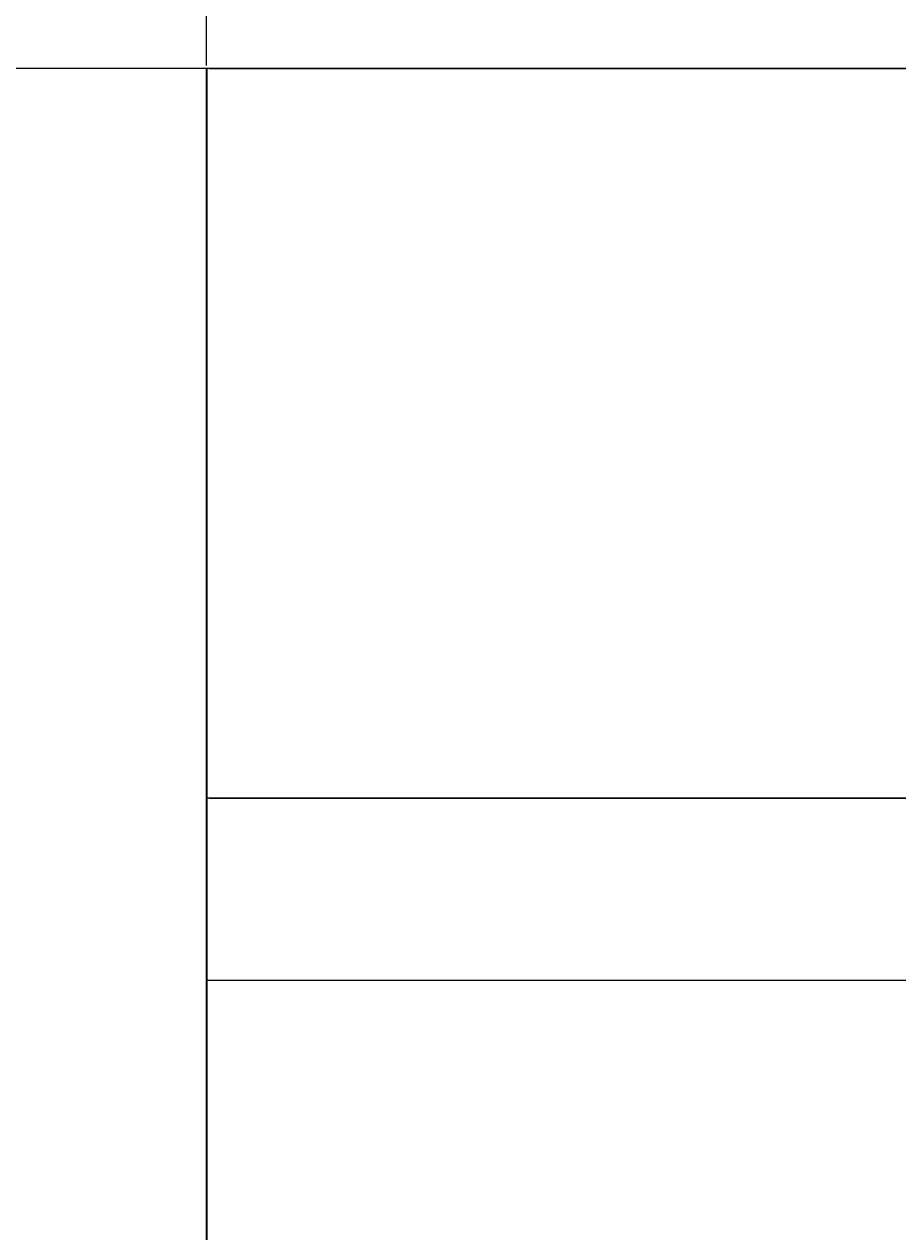
# Model space of a CAD drawing. Units: feet. Extents: x 105 to 1094, y -88 to 588.
# Tile 31 of 59: x 346 to 365, y 518 to 544. Entities that reach past the tile are written whole.
import ezdxf

# ---------------------------------------------------------------- set-up
doc = ezdxf.new("R2010")
doc.units = ezdxf.units.FT
doc.header["$MEASUREMENT"] = 0
for name, color, linetype, lineweight in [('A-ANNO-DIMS', 2, 'Continuous', 18), ('A-FLOR-PROJ', 8, 'Continuous', 25), ('A-WALL', 7, 'Continuous', 35)]:
    doc.layers.add(name, color=color, linetype=linetype, lineweight=lineweight)
doc.styles.get("Standard").update_dxf_attribs({"font": 'arial.ttf'})
doc.dimstyles.get("Standard").update_dxf_attribs({"dimtxt": 0.18, "dimasz": 0.18, "dimexe": 0.18, "dimexo": 0.0625, "dimgap": 0.09, "dimtad": 0, "dimtih": 1, "dimtoh": 1, "dimdec": 4, "dimzin": 0, "dimdsep": 46, "dimtxsty": 'Standard', "dimcen": 0.09, "dimadec": 0, "dimazin": 0, "dimtfac": 1, "dimtdec": 4, "dimtofl": 0, "dimtmove": 0, "dimatfit": 3, "dimfxl": 1, "dimtolj": 1, "dimtzin": 0, "dimarcsym": 0})

# ---------------------------------------------------------------- blocks, each defined once
blk = doc.blocks.new('*D21')
at = {"layer": 'A-ANNO-DIMS', "color": 0, "lineweight": -2, "transparency": 16777216}
for p, q in [((849.626, 543.081), (105.458, 543.081)), ((105.638, 542.901), (105.638, 250.263)), ((105.638, -42.739), (105.638, 249.899)), ((849.626, -42.919), (105.458, -42.919))]:
    blk.add_line(p, q, dxfattribs=at)
at = {"layer": 'A-ANNO-DIMS', "color": 0, "transparency": 16777216}
for points in [[(105.608, 542.901), (105.668, 542.901), (105.638, 543.081)], [(105.608, -42.739), (105.668, -42.739), (105.638, -42.919)]]:
    blk.add_solid(points, dxfattribs=at)
at = {"layer": 'Defpoints', "color": 0, "transparency": 16777216}
for p in [(105.638, 543.081), (849.688, 543.081), (849.688, -42.919)]:
    blk.add_point(p, dxfattribs=at)
at = {"layer": 'A-ANNO-DIMS', "color": 0, "transparency": 16777216, "insert": (105.638, 250.081), "char_height": 0.18, "attachment_point": 5}
blk.add_mtext('\\A1;586', dxfattribs=at)
blk = doc.blocks.new('*D23')
at = {"layer": 'A-ANNO-DIMS', "color": 0, "lineweight": -2, "transparency": 16777216}
for p, q in [((231.688, 543.144), (231.688, 588.311)), ((349.688, 543.144), (349.688, 588.311)), ((231.868, 588.131), (290.408, 588.131)), ((349.508, 588.131), (290.969, 588.131))]:
    blk.add_line(p, q, dxfattribs=at)
at = {"layer": 'A-ANNO-DIMS', "color": 0, "transparency": 16777216}
for points in [[(231.868, 588.161), (231.868, 588.101), (231.688, 588.131)], [(349.508, 588.161), (349.508, 588.101), (349.688, 588.131)]]:
    blk.add_solid(points, dxfattribs=at)
at = {"layer": 'Defpoints', "color": 0, "transparency": 16777216}
for p in [(349.688, 588.131), (231.688, 543.081), (349.688, 543.081)]:
    blk.add_point(p, dxfattribs=at)
at = {"layer": 'A-ANNO-DIMS', "color": 0, "transparency": 16777216, "insert": (290.688, 588.131), "char_height": 0.18, "attachment_point": 5}
blk.add_mtext('\\A1;118', dxfattribs=at)
blk = doc.blocks.new('*D24')
at = {"layer": 'A-ANNO-DIMS', "color": 0, "lineweight": -2, "transparency": 16777216}
for p, q in [((349.688, 543.144), (349.688, 588.311)), ((438.688, 527.144), (438.688, 588.311)), ((349.868, 588.131), (393.969, 588.131)), ((438.508, 588.131), (394.408, 588.131))]:
    blk.add_line(p, q, dxfattribs=at)
at = {"layer": 'A-ANNO-DIMS', "color": 0, "transparency": 16777216}
for points in [[(349.868, 588.161), (349.868, 588.101), (349.688, 588.131)], [(438.508, 588.161), (438.508, 588.101), (438.688, 588.131)]]:
    blk.add_solid(points, dxfattribs=at)
at = {"layer": 'Defpoints', "color": 0, "transparency": 16777216}
for p in [(438.688, 588.131), (349.688, 543.081), (438.688, 527.081)]:
    blk.add_point(p, dxfattribs=at)
at = {"layer": 'A-ANNO-DIMS', "color": 0, "transparency": 16777216, "insert": (394.188, 588.131), "char_height": 0.18, "attachment_point": 5}
blk.add_mtext('\\A1;89', dxfattribs=at)
blk = doc.blocks.new('*D30')
at = {"layer": 'A-ANNO-DIMS', "color": 0, "lineweight": -2, "transparency": 16777216}
for p, q in [((349.751, 543.081), (1093.918, 543.081)), ((1093.738, 542.901), (1093.738, 535.263)), ((1093.738, 527.261), (1093.738, 534.899)), ((349.751, 527.081), (1093.918, 527.081))]:
    blk.add_line(p, q, dxfattribs=at)
at = {"layer": 'A-ANNO-DIMS', "color": 0, "transparency": 16777216}
for points in [[(1093.708, 542.901), (1093.768, 542.901), (1093.738, 543.081)], [(1093.708, 527.261), (1093.768, 527.261), (1093.738, 527.081)]]:
    blk.add_solid(points, dxfattribs=at)
at = {"layer": 'Defpoints', "color": 0, "transparency": 16777216}
for p in [(349.688, 543.081), (349.688, 527.081), (1093.738, 527.081)]:
    blk.add_point(p, dxfattribs=at)
at = {"layer": 'A-ANNO-DIMS', "color": 0, "transparency": 16777216, "insert": (1093.738, 535.081), "char_height": 0.18, "attachment_point": 5}
blk.add_mtext('\\A1;16', dxfattribs=at)
blk = doc.blocks.new('*D39')
at = {"layer": 'A-ANNO-DIMS', "color": 0, "lineweight": -2, "transparency": 16777216}
for p, q in [((294.688, 204.144), (294.688, 588.311)), ((370.688, 204.144), (370.688, 588.311)), ((294.868, 588.131), (332.47, 588.131)), ((370.508, 588.131), (332.906, 588.131))]:
    blk.add_line(p, q, dxfattribs=at)
at = {"layer": 'A-ANNO-DIMS', "color": 0, "transparency": 16777216}
for points in [[(294.868, 588.161), (294.868, 588.101), (294.688, 588.131)], [(370.508, 588.161), (370.508, 588.101), (370.688, 588.131)]]:
    blk.add_solid(points, dxfattribs=at)
at = {"layer": 'Defpoints', "color": 0, "transparency": 16777216}
for p in [(370.688, 588.131), (294.688, 204.081), (370.688, 204.081)]:
    blk.add_point(p, dxfattribs=at)
at = {"layer": 'A-ANNO-DIMS', "color": 0, "transparency": 16777216, "insert": (332.688, 588.131), "char_height": 0.18, "attachment_point": 5}
blk.add_mtext('\\A1;76', dxfattribs=at)

msp = doc.modelspace()

# ---------------------------------------------------------------- linework, layer by layer
at = {"layer": 'A-FLOR-PROJ'}
for p, q in [((349.6883, 543.0812), (231.6883, 543.0812)), ((438.6883, 527.0812), (349.6883, 527.0812)), ((434.6883, 523.0812), (349.6883, 523.0812))]:
    msp.add_line(p, q, dxfattribs=at)
at = {"layer": 'A-WALL'}
msp.add_line((349.6883, 543.0812), (349.6883, 497.0812), dxfattribs=at)

# ---------------------------------------------------------------- dimensions: what is measured, and where the dimension line sits
at = {"layer": 'A-ANNO-DIMS'}
for base, p1, p2, picture, middle in [((349.6883, 588.1312), (231.6883, 543.0812), (349.6883, 543.0812), '*D23', (290.6883, 588.1312)), ((370.6883, 588.1312), (294.6883, 204.0812), (370.6883, 204.0812), '*D39', (332.6883, 588.1312)), ((438.6883, 588.1312), (349.6883, 543.0812), (438.6883, 527.0812), '*D24', (394.1883, 588.1312))]:
    dim = msp.add_linear_dim(base=base, p1=p1, p2=p2, dimstyle='Standard', override={"dimdec": 0, "dimlfac": 1, "dimrnd": 0, "dimzin": 0, "dimdsep": 46, "dimlunit": 2}, dxfattribs=at)
    dim.commit()
    dim.dimension.update_dxf_attribs({"geometry": picture, "text_midpoint": middle})
for base, p1, p2, picture, middle in [((105.6383, 543.0812), (849.6883, -42.9188), (849.6883, 543.0812), '*D21', (105.6383, 250.0812)), ((1093.7383, 527.0812), (349.6883, 543.0812), (349.6883, 527.0812), '*D30', (1093.7383, 535.0812))]:
    dim = msp.add_linear_dim(base=base, p1=p1, p2=p2, angle=90, dimstyle='Standard', override={"dimdec": 0, "dimlfac": 1, "dimrnd": 0, "dimzin": 0, "dimdsep": 46, "dimlunit": 2}, dxfattribs=at)
    dim.commit()
    dim.dimension.update_dxf_attribs({"geometry": picture, "text_midpoint": middle})

doc.saveas('drawing.dxf')
